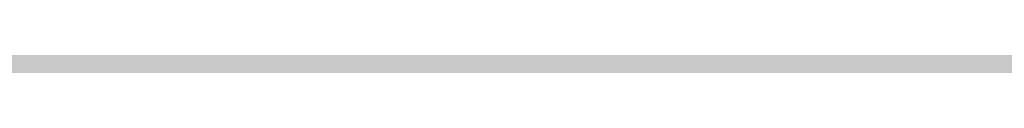
# Model space of a CAD drawing. Units: inches. Extents: x 2091 to 2899, y 967 to 2217.
# Tile 212 of 256: x 2203.2571 to 2203.4104, y 1152.2475 to 1152.2479. Entities that reach past the tile are written whole.
import ezdxf

# ---------------------------------------------------------------- set-up
doc = ezdxf.new("R2010")
doc.units = ezdxf.units.IN
doc.layers.add('A-WALL-PATT', color=141, linetype='Continuous', lineweight=13, true_color=0xadddf7)

msp = doc.modelspace()

# ---------------------------------------------------------------- hatches: boundary and pattern name
at = {"layer": 'A-WALL-PATT'}
h = msp.add_hatch(color=256, dxfattribs=at)
h.dxf.hatch_style = 1
h.paths.add_polyline_path([(2803.1436, 2050.91906), (2203.1436, 2050.91906), (2203.1436, 1090.91906), (2803.1436, 1090.91906)])
h.paths.add_polyline_path([(2635.79885, 1147.54046), (2674.52405, 1147.54046, 0.376086), (2678.52967, 1152.8802), (2678.52967, 1159.55647, 0.333335), (2674.52432, 1163.56185), (2674.52432, 1163.56185), (2674.52432, 1192.93439), (2635.80597, 1192.93439), (2597.08762, 1192.93439), (2597.08762, 1163.56185, 0.333335), (2593.08228, 1159.55647), (2593.08228, 1152.8802, 0.376086), (2597.08789, 1147.54046)], flags=0)
h.paths.add_polyline_path([(2436.01043, 1278.24078, 0.000483), (2435.95264, 1278.21503, -0.001328), (2435.93563, 1278.11169, -0.001711), (2436.11644, 1278.04076, 0.002185)], flags=0)
h.paths.add_polyline_path([(2794.1436, 1143.41906), (2794.1436, 1347.41906), (2543.37017, 1347.41906), (2543.37017, 1351.91906), (2794.1436, 1351.91906), (2794.1436, 1392.71355), (2793.9474, 1392.71355), (2793.9474, 1473.5369), (2794.1436, 1473.5369), (2794.1436, 1531.91906), (2650.1436, 1531.91906), (2650.1436, 1536.41906), (2794.1436, 1536.41906), (2794.1436, 1692.41906), (2609.37561, 1692.41906), (2609.37561, 1644.41906), (2604.87561, 1644.41906), (2604.87561, 1744.91906), (2609.37561, 1744.91906), (2609.37561, 1696.91906), (2794.1436, 1696.91906), (2794.1436, 1780.91906), (2609.6436, 1780.91906), (2493.87561, 1780.91906), (2493.87561, 1785.41906), (2609.6436, 1785.41906), (2794.1436, 1785.41906), (2794.1436, 1847.93882), (2793.95122, 1847.93882), (2793.95122, 1928.76217), (2794.1436, 1928.76217), (2794.1436, 1941.41906), (2614.1436, 1941.41906), (2614.1436, 1821.41906), (2609.6436, 1821.41906), (2609.6436, 1941.41906), (2392.1436, 1941.41906), (2392.1436, 1819.91906), (2387.6436, 1819.91906), (2387.6436, 1941.41906), (2212.1436, 1941.41906), (2212.1436, 1783.91906), (2392.1436, 1783.91906), (2392.1436, 1780.91906), (2212.1436, 1780.91906), (2212.1436, 1629.41906), (2387.6436, 1629.41906), (2387.6436, 1744.91906), (2392.1436, 1744.91906), (2392.1436, 1627.91906), (2317.1436, 1627.91906), (2317.1436, 1551.41906), (2317.1436, 1536.41906), (2459.38359, 1536.41906), (2459.38359, 1602.39648), (2463.88359, 1602.39648), (2463.88359, 1531.91906), (2456.6436, 1531.91906), (2456.6436, 1529.91906), (2452.1436, 1529.91906), (2452.1436, 1531.91906), (2312.6436, 1531.91906), (2312.6436, 1551.41906), (2306.1436, 1551.41906), (2306.1436, 1555.91906), (2308.1436, 1555.91906), (2308.1436, 1551.41906), (2312.6436, 1551.41906), (2312.6436, 1627.91906), (2212.1436, 1627.91906), (2212.1436, 1555.91906), (2270.1436, 1555.91906), (2270.1436, 1551.41906), (2212.1436, 1551.41906), (2212.1436, 1351.91906), (2272.1436, 1351.91906), (2272.1436, 1347.41906), (2212.1436, 1347.41906), (2212.1436, 1275.41906), (2308.1436, 1275.41906), (2308.1436, 1351.91906), (2452.1436, 1351.91906), (2452.1436, 1493.91906), (2456.6436, 1493.91906), (2456.6436, 1347.41906), (2312.6436, 1347.41906), (2312.6436, 1270.91906), (2212.1436, 1270.91906), (2212.1436, 1099.91906), (2281.23752, 1099.91906), (2282.87104, 1110.9138), (2282.00834, 1116.9966), (2278.55774, 1121.4204), (2268.20564, 1128.0562), (2272.08764, 1128.0562), (2273.81294, 1131.927), (2279.42034, 1134.6919), (2285.02784, 1135.2449), (2287.61584, 1137.4568), (2288.04714, 1138.0098), (2289.34114, 1140.7747), (2291.06654, 1139.6687), (2292.36054, 1135.2449), (2295.37984, 1136.9038), (2296.24254, 1135.7979), (2297.10524, 1133.033), (2300.12464, 1138.0098), (2303.14394, 1138.0098), (2304.43794, 1135.7979), (2303.14394, 1133.586), (2306.59464, 1134.6919), (2307.88874, 1133.033), (2310.90804, 1135.2449), (2313.92744, 1134.1389), (2315.62686, 1132.4271), (2308.32004, 1117.5496), (2290.20384, 1109.8079), (2288.90984, 1103.1721), (2289.27231, 1099.91906), (2434.91823, 1099.91906), (2431.59323, 1124.78806), (2429.93023, 1169.55306), (2430.92718, 1240.51969), (2435.65893, 1238.18613), (2437.13523, 1196.55406), (2438.79823, 1143.97306), (2442.67823, 1111.99806), (2446.55823, 1099.91906), (2794.1436, 1099.91906), (2794.1436, 1138.91906), (2548.03245, 1138.91906), (2548.03245, 1143.41906), (2548.03245, 1148.81906), (2546.66846, 1148.03156), (2528.68569, 1179.17862, 0.256256), (2512.03245, 1148.81906), (2512.03245, 1143.41906), (2512.03245, 1138.91906), (2507.53245, 1138.91906), (2507.53245, 1143.41906), (2507.53245, 1148.81906, 0.256256), (2490.8792, 1179.17862), (2472.89644, 1148.03156), (2471.53245, 1148.81906), (2471.53245, 1143.41906), (2467.03245, 1143.41906), (2467.03245, 1269.94579, 0.039061), (2460.90999, 1273.58006), (2467.03245, 1273.58006), (2467.03245, 1286.32536, 0.014511), (2465.21619, 1286.76191), (2467.03245, 1287.05258), (2467.03245, 1323.41906), (2471.53245, 1323.41906), (2471.53245, 1148.81906), (2489.53245, 1179.99597), (2490.89644, 1179.20847), (2490.8792, 1179.17862, -0.256256), (2507.53245, 1148.81906), (2507.53245, 1143.41906), (2512.03245, 1143.41906), (2512.03245, 1148.81906, -0.256256), (2528.68569, 1179.17862), (2528.66846, 1179.20847), (2530.03245, 1179.99597), (2548.03245, 1148.81906), (2548.03245, 1143.41906)], flags=16)
h.paths.add_polyline_path([(2607.76855, 1200.94508), (2607.76855, 1265.03063), (2597.08762, 1281.05201), (2619.78459, 1281.05201), (2627.79528, 1337.12686), (2635.79885, 1337.12686), (2643.81666, 1337.12686), (2651.82736, 1281.05201), (2674.52432, 1281.05201), (2663.8434, 1265.03063), (2663.8434, 1200.94508), (2635.80597, 1200.94508)], flags=0)
edge = h.paths.add_edge_path(flags=0)
edge.add_ellipse((13303.89622, 1272.99872), major_axis=(-10595.31304, 0), ratio=0.84230387009, start_angle=0.628237219, end_angle=0.6465541, ccw=False)
edge.add_ellipse((2711.70045, 1156.85268), major_axis=(2.21977, 0), ratio=0.8423039, start_angle=111.53524, end_angle=180.62824, ccw=False)
edge.add_ellipse((13303.15629, 1272.99872), major_axis=(-10593.02631, 0), ratio=0.84230386954, start_angle=0.528271472, end_angle=0.646554097, ccw=False)
edge.add_line((2710.7646, 1175.3333), (2710.12999, 1175.3333))
edge.add_ellipse((2710.12999, 1176.57978), major_axis=(1.47985, 0), ratio=0.8423039, start_angle=180, end_angle=270, ccw=False)
edge.add_line((2708.65014, 1176.57978), (2708.65014, 1200.78291))
edge.add_ellipse((2710.12999, 1200.78291), major_axis=(1.47985, 0), ratio=0.8423039, start_angle=90, end_angle=180, ccw=False)
edge.add_line((2710.12999, 1202.02939), (2710.46508, 1202.02939))
edge.add_ellipse((13303.15629, 1272.99872), major_axis=(-10593.02631, 0), ratio=0.84230386954, start_angle=-0.090229089, end_angle=0.383866779, ccw=False)
edge.add_ellipse((2710.12999, 1290.92703), major_axis=(-1.47985, 0), ratio=0.8423039, start_angle=0, end_angle=90, ccw=False)
edge.add_line((2708.65014, 1290.92703), (2708.65014, 1315.13017))
edge.add_ellipse((2710.12999, 1315.13017), major_axis=(-1.47985, 0), ratio=0.8423039, start_angle=-90, end_angle=0, ccw=False)
edge.add_line((2710.12999, 1316.37665), (2710.70631, 1316.37665))
edge.add_ellipse((3238.40172, 1296.28957), major_axis=(528.234, 0), ratio=0.84230387, start_angle=176.3495724, end_angle=177.8200497, ccw=False)
edge.add_ellipse((2775.06304, 1071.4507), major_axis=(313.30776, 0), ratio=0.84230387, start_angle=102.1259656, end_angle=103.780529, ccw=False)
edge.add_ellipse((2775.06304, 1078.3057), major_axis=(-305.30289, 0), ratio=0.84230387, start_angle=-79.790461, end_angle=-77.5553727, ccw=False)
edge.add_ellipse((2695.14177, 1541.97538), major_axis=(-250.96022, 0), ratio=0.84230387, start_angle=99.256566, end_angle=102.5549326)
edge.add_line((2741.41033, 1334.21426), (2747.13255, 1337.37848))
edge.add_ellipse((2747.53862, 1336.85748), major_axis=(-0.73992, 0), ratio=0.842304, start_angle=270, end_angle=307.93313, ccw=False)
edge.add_ellipse((2747.53862, 1336.85748), major_axis=(-0.73992, 0), ratio=0.842304, start_angle=232.06687, end_angle=270, ccw=False)
edge.add_line((2747.94469, 1337.37848), (2753.66691, 1334.21426))
edge.add_ellipse((2799.93547, 1541.97538), major_axis=(250.96022, 0), ratio=0.84230387, start_angle=257.4450674, end_angle=260.743434)
edge.add_ellipse((2720.01419, 1078.3057), major_axis=(305.30289, 0), ratio=0.84230387, start_angle=77.5553727, end_angle=79.790461, ccw=False)
edge.add_ellipse((2720.01419, 1071.4507), major_axis=(-313.30776, 0), ratio=0.84230387, start_angle=256.219471, end_angle=257.8740344, ccw=False)
edge.add_ellipse((2256.67551, 1296.28957), major_axis=(-528.234, 0), ratio=0.84230387, start_angle=182.1799503, end_angle=183.6504276, ccw=False)
edge.add_line((2784.37092, 1316.37665), (2784.94725, 1316.37665))
edge.add_ellipse((2784.94725, 1315.13017), major_axis=(1.47985, 0), ratio=0.8423039, start_angle=0, end_angle=90, ccw=False)
edge.add_line((2786.42709, 1315.13017), (2786.42709, 1290.92703))
edge.add_ellipse((2784.94725, 1290.92703), major_axis=(1.47985, 0), ratio=0.8423039, start_angle=270, end_angle=360, ccw=False)
edge.add_ellipse((-7808.07906, 1272.99872), major_axis=(10593.02631, 0), ratio=0.84230386954, start_angle=-0.383866779, end_angle=0.090229089, ccw=False)
edge.add_line((2784.61216, 1202.02939), (2784.94725, 1202.02939))
edge.add_ellipse((2784.94725, 1200.78291), major_axis=(1.47985, 0), ratio=0.8423039, start_angle=0, end_angle=90, ccw=False)
edge.add_line((2786.42709, 1200.78291), (2786.42709, 1176.57978))
edge.add_ellipse((2784.94725, 1176.57978), major_axis=(-1.47985, 0), ratio=0.8423039, start_angle=90, end_angle=180, ccw=False)
edge.add_line((2784.94725, 1175.3333), (2784.31264, 1175.3333))
edge.add_ellipse((-7808.07906, 1272.99872), major_axis=(10593.02631, 0), ratio=0.84230386954, start_angle=-0.618643196, end_angle=-0.528271472, ccw=False)
edge.add_ellipse((2783.37678, 1156.85268), major_axis=(-2.21977, 0), ratio=0.8423039, start_angle=179.37176, end_angle=248.46476, ccw=False)
edge.add_ellipse((-7808.81898, 1272.99872), major_axis=(-10595.31304, 0), ratio=0.84230386576, start_angle=179.353445923, end_angle=179.371762803, ccw=False)
edge.add_ellipse((2780.2973, 1153.50079), major_axis=(-5.24643, 0), ratio=0.8423039, start_angle=90, end_angle=179.35345, ccw=False)
edge.add_line((2780.2973, 1149.08171), (2714.77993, 1149.08171))
edge.add_ellipse((2714.77993, 1153.50079), major_axis=(5.24643, 0), ratio=0.8423039, start_angle=180.64655, end_angle=270, ccw=False)
edge = h.paths.add_edge_path(flags=0)
edge.add_line((2718.18737, 1151.00783), (2718.18737, 1170.47236))
edge.add_ellipse((2721.14706, 1170.47236), major_axis=(-2.95969, 0), ratio=0.8423039, start_angle=-90, end_angle=0, ccw=False)
edge.add_line((2721.14706, 1172.96532), (2773.93017, 1172.96532))
edge.add_ellipse((2773.93017, 1170.47236), major_axis=(-2.95969, 0), ratio=0.8423039, start_angle=180, end_angle=270, ccw=False)
edge.add_line((2776.88987, 1170.47236), (2776.88987, 1151.00783))
edge.add_line((2776.88987, 1151.00783), (2718.18737, 1151.00783))
edge = h.paths.add_edge_path(flags=0)
edge.add_line((2718.18737, 1180.23415), (2718.18737, 1199.05783))
edge.add_ellipse((2747.53862, 1320.39864), major_axis=(147.01792, 0), ratio=0.84230387, start_angle=256.4018653, end_angle=283.5981347)
edge.add_line((2776.88987, 1199.05783), (2776.88987, 1180.23415))
edge.add_ellipse((2747.53862, 1301.57496), major_axis=(147.01792, 0), ratio=0.84230387, start_angle=256.4018653, end_angle=283.5981347, ccw=False)
edge = h.paths.add_edge_path(flags=0)
edge.add_ellipse((13303.15629, 1272.99872), major_axis=(-10591.54646, 0), ratio=0.84230386955, start_angle=0.055594314, end_angle=0.377764194, ccw=False)
edge.add_line((2711.61686, 1262.72171), (2715.66741, 1249.4954))
edge.add_ellipse((6413.89196, 1241.69192), major_axis=(-3698.23616, 0), ratio=0.8423038695, start_angle=-0.12089737, end_angle=0.36407635)
edge.add_line((2715.76104, 1218.19245), (2711.93431, 1203.16736))
edge = h.paths.add_edge_path(flags=0)
edge.add_line((2718.18737, 1251.07457), (2716.00249, 1267.45044))
edge.add_ellipse((2742.15117, 1202.18954), major_axis=(81.77258, 0), ratio=0.84230387, start_angle=94.277421, end_angle=111.8349538, ccw=False)
edge.add_line((2737.00975, 1270.93063), (2758.06748, 1270.93063))
edge.add_ellipse((2752.92606, 1202.18954), major_axis=(81.77258, 0), ratio=0.84230387, start_angle=68.1650462, end_angle=85.722579, ccw=False)
edge.add_line((2779.07475, 1267.45044), (2776.88987, 1251.07457))
edge.add_ellipse((2750.33806, 1187.88536), major_axis=(79.57966, 0), ratio=0.84230387, start_angle=67.2080851, end_angle=85.1299304)
edge.add_line((2756.03466, 1254.74366), (2739.04258, 1254.74366))
edge.add_ellipse((2744.73917, 1187.88536), major_axis=(79.57966, 0), ratio=0.84230387, start_angle=94.8700696, end_angle=112.7919149)
edge = h.paths.add_edge_path(flags=0)
edge.add_line((2783.14293, 1203.16736), (2779.31619, 1218.19245))
edge.add_ellipse((-918.81473, 1241.69192), major_axis=(3698.23616, 0), ratio=0.8423038695, start_angle=-0.36407635, end_angle=0.12089737)
edge.add_line((2779.40983, 1249.4954), (2783.46037, 1262.72171))
edge.add_ellipse((-7808.07906, 1272.99872), major_axis=(-10591.54646, 0), ratio=0.84230386954, start_angle=179.622235806, end_angle=179.944405687, ccw=False)
edge = h.paths.add_edge_path(flags=0)
edge.add_ellipse((2734.20089, 1286.69044), major_axis=(-0.35661, 6.34008), ratio=0.6038336, start_angle=89.002014, end_angle=253.657408, ccw=False)
edge.add_line((2730.369, 1286.54181), (2730.369, 1301.35198))
edge.add_line((2730.369, 1301.35198), (2735.91331, 1305.2148))
edge.add_ellipse((2736.38492, 1304.73456), major_axis=(0.73992, 0), ratio=0.842304, start_angle=90, end_angle=134.48021, ccw=False)
edge.add_line((2736.38492, 1305.3578), (2738.03278, 1305.3578))
edge.add_line((2738.03278, 1305.3578), (2738.03278, 1307.70793))
edge.add_ellipse((2794.20164, 1307.70793), major_axis=(56.16886, 0), ratio=0.84230387, start_angle=150.56143, end_angle=180, ccw=False)
edge.add_ellipse((2700.87559, 1307.70793), major_axis=(-56.16886, 0), ratio=0.84230387, start_angle=180, end_angle=209.43857, ccw=False)
edge.add_line((2757.04445, 1307.70793), (2757.04445, 1305.3578))
edge.add_line((2757.04445, 1305.3578), (2758.69232, 1305.3578))
edge.add_ellipse((2758.69232, 1304.73456), major_axis=(-0.73992, 0), ratio=0.842304, start_angle=225.51979, end_angle=270, ccw=False)
edge.add_line((2759.16392, 1305.2148), (2764.70823, 1301.35198))
edge.add_line((2764.70823, 1301.35198), (2764.70823, 1286.54181))
edge.add_ellipse((2760.87634, 1286.69044), major_axis=(0.35661, 6.34008), ratio=0.6038336, start_angle=106.342592, end_angle=270.997986, ccw=False)
edge.add_line((2757.04445, 1285.79709), (2757.04445, 1307.70793))
edge.add_ellipse((2700.87559, 1307.70793), major_axis=(-56.16886, 0), ratio=0.84230387, start_angle=180, end_angle=209.43857)
edge.add_ellipse((2794.20164, 1307.70793), major_axis=(56.16886, 0), ratio=0.84230387, start_angle=150.56143, end_angle=180)
edge.add_line((2738.03278, 1307.70793), (2738.03278, 1285.79709))
h.paths.add_polyline_path([(2417.81227, 1104.4497), (2413.49227, 1102.5297), (2410.61227, 1103.9697), (2409.17227, 1106.3697), (2407.25227, 1107.3297), (2406.29227, 1109.7297), (2405.33227, 1114.0497), (2405.33227, 1117.8897), (2406.29227, 1120.1297), (2407.25227, 1119.8097), (2408.84832, 1118.32766), (2410.17395, 1119.42417), (2410.21127, 1120.4057), (2411.04073, 1121.41905), (2410.69927, 1119.8587), (2410.17395, 1119.42417), (2410.08845, 1117.17611), (2411.13284, 1116.20632), (2413.97227, 1119.3297), (2416.85227, 1120.7697), (2416.86972, 1120.79878), (2417.03507, 1119.40512), (2417.89621, 1118.14338), (2418.29227, 1118.3697), (2419.54445, 1120.03927), (2419.36092, 1118.38749), (2419.03211, 1119.35615), (2418.39894, 1118.51193), (2419.25227, 1114.5297), (2418.79409, 1107.19879)], flags=0)
h.paths.add_polyline_path([(2508.87017, 1347.41906), (2508.37017, 1347.41906), (2508.37017, 1351.91906), (2508.87017, 1351.91906)], flags=0)
h.paths.add_polyline_path([(2473.37017, 1347.41906), (2472.37017, 1347.41906), (2467.87017, 1347.41906), (2467.87017, 1455.41906), (2472.37017, 1455.41906), (2472.37017, 1352.41906), (2473.37017, 1352.41906)], flags=0)
h.paths.add_polyline_path([(2352.10624, 1217.4462), (2349.22624, 1218.8862), (2347.78624, 1221.2862), (2345.86624, 1222.2462), (2344.90624, 1224.6462), (2343.94624, 1228.9662), (2343.94624, 1232.8062), (2344.90624, 1235.0462), (2345.86624, 1234.7262), (2347.46229, 1233.24415), (2348.78792, 1234.34066), (2348.82524, 1235.3222), (2349.6547, 1236.33555), (2349.31324, 1234.7752), (2348.78792, 1234.34066), (2348.70242, 1232.0926), (2349.74681, 1231.12282), (2352.58624, 1234.2462), (2355.46624, 1235.6862), (2355.48369, 1235.71528), (2355.64904, 1234.32161), (2356.51018, 1233.05988), (2356.90624, 1233.2862), (2358.15842, 1234.95576), (2357.97489, 1233.30398), (2357.64608, 1234.27264), (2357.01291, 1233.42842), (2357.86624, 1229.4462), (2357.40806, 1222.11529), (2356.42624, 1219.3662)], flags=0)
h.paths.add_polyline_path([(2348.2968, 1112.22442), (2347.0138, 1112.31042), (2345.5298, 1114.12742), (2345.7318, 1115.85842), (2346.8118, 1116.98242), (2346.8118, 1114.64642), (2345.8668, 1114.21442), (2346.8798, 1114.30042)], flags=0)
h.paths.add_polyline_path([(2347.0138, 1110.92642), (2346.2718, 1110.49342), (2346.6098, 1111.18642)], flags=0)
h.paths.add_polyline_path([(2345.8668, 1118.19442), (2345.5298, 1117.32942), (2343.7078, 1118.02142), (2344.3828, 1118.62642)], flags=0)
h.paths.add_polyline_path([(2346.6768, 1109.28242), (2346.0698, 1108.07142), (2345.8668, 1110.06142)], flags=0)
h.paths.add_polyline_path([(2345.0568, 1119.75142), (2343.6398, 1119.75142), (2343.9778, 1121.13542)], flags=0)
h.paths.add_polyline_path([(2345.2598, 1116.55042), (2345.1248, 1115.85842), (2344.9218, 1115.68542), (2344.7198, 1116.37742)], flags=0)
h.paths.add_polyline_path([(2345.6648, 1112.31042), (2345.4618, 1111.53242), (2344.0448, 1111.96442), (2344.6518, 1112.57042)], flags=0)
h.paths.add_polyline_path([(2345.1918, 1113.34942), (2344.4498, 1113.86842), (2344.7198, 1114.38742)], flags=0)
h.paths.add_polyline_path([(2344.6518, 1116.80942), (2344.1798, 1115.68542), (2344.6518, 1115.33942), (2343.9098, 1114.90642), (2343.0328, 1115.94442), (2343.6398, 1116.46342)], flags=0)
h.paths.add_polyline_path([(2345.8668, 1106.68642), (2344.9898, 1105.56242), (2344.5168, 1106.60042)], flags=0)
h.paths.add_polyline_path([(2344.8548, 1110.06142), (2344.5168, 1109.28242), (2344.1128, 1109.71542)], flags=0)
h.paths.add_polyline_path([(2344.0448, 1113.52242), (2343.4378, 1113.08942), (2342.7628, 1113.95442)], flags=0)
h.paths.add_polyline_path([(2344.3148, 1111.01242), (2342.9648, 1110.32042), (2342.9648, 1111.09942)], flags=0)
h.paths.add_polyline_path([(2345.1248, 1104.69742), (2344.5848, 1103.74542), (2344.4498, 1104.26442)], flags=0)
h.paths.add_polyline_path([(2342.8298, 1121.22242), (2341.7498, 1120.53042), (2340.5358, 1121.04942), (2340.1308, 1121.82842), (2340.6708, 1122.95242), (2341.1428, 1121.82842), (2341.6148, 1122.00142)], flags=0)
h.paths.add_polyline_path([(2342.9648, 1119.75142), (2343.0328, 1118.45342), (2342.0878, 1118.02142), (2342.0198, 1119.49142)], flags=0)
h.paths.add_polyline_path([(2342.6948, 1116.89642), (2341.9528, 1116.63642), (2342.0198, 1117.32942)], flags=0)
h.paths.add_polyline_path([(2343.0328, 1112.22442), (2342.0198, 1111.79142), (2341.5478, 1112.22442), (2342.3578, 1113.34942)], flags=0)
h.paths.add_polyline_path([(2343.7748, 1104.43742), (2342.6278, 1102.88042), (2342.6948, 1104.61042), (2343.4378, 1105.12942)], flags=0)
h.paths.add_polyline_path([(2342.0198, 1115.07942), (2340.8058, 1115.51242), (2340.9408, 1116.37742)], flags=0)
h.paths.add_polyline_path([(2341.4808, 1120.09742), (2341.4808, 1119.40542), (2341.0758, 1119.57842), (2341.1428, 1120.09742)], flags=0)
h.paths.add_polyline_path([(2341.8178, 1114.47342), (2340.9408, 1113.08942), (2340.8058, 1114.56042)], flags=0)
h.paths.add_polyline_path([(2341.1428, 1118.54042), (2340.9408, 1116.98242), (2339.0508, 1117.67542), (2339.0508, 1118.62642)], flags=0)
h.paths.add_polyline_path([(2342.6948, 1101.66842), (2341.9528, 1101.84142), (2342.5598, 1102.36142)], flags=0)
h.paths.add_polyline_path([(2340.3328, 1119.66542), (2338.4438, 1119.57842), (2337.9038, 1120.35742), (2339.6578, 1120.61642)], flags=0)
h.paths.add_polyline_path([(2340.3328, 1115.33942), (2340.0628, 1113.69542), (2339.3878, 1115.33942)], flags=0)
h.paths.add_polyline_path([(2341.8178, 1103.83142), (2341.5478, 1102.88042), (2341.1428, 1103.65842)], flags=0)
h.paths.add_polyline_path([(2339.0508, 1122.86642), (2337.2958, 1121.82842), (2337.0938, 1123.12542), (2337.7688, 1123.81842)], flags=0)
h.paths.add_polyline_path([(2339.1178, 1121.74142), (2338.8478, 1121.22242), (2338.1738, 1121.04942), (2338.3758, 1121.56842)], flags=0)
h.paths.add_polyline_path([(2339.1858, 1119.31942), (2338.6458, 1118.71342), (2338.2408, 1118.10742), (2338.2408, 1118.88642)], flags=0)
h.paths.add_polyline_path([(2341.1428, 1101.92842), (2340.6028, 1101.23642), (2340.0628, 1101.84142), (2340.6028, 1102.36142)], flags=0)
h.paths.add_polyline_path([(2337.6338, 1117.76142), (2336.6208, 1118.28042), (2337.2958, 1118.97242)], flags=0)
h.paths.add_polyline_path([(2336.8238, 1119.57842), (2334.7988, 1118.97242), (2335.2038, 1120.35742), (2336.5538, 1120.87642)], flags=0)
h.paths.add_polyline_path([(2339.1178, 1100.45742), (2337.3638, 1100.54342), (2336.7558, 1101.23642)], flags=0)
h.paths.add_polyline_path([(2336.3508, 1122.43342), (2336.0138, 1121.91442), (2334.9338, 1122.43342), (2334.5288, 1123.47142), (2335.7438, 1122.77942)], flags=0)
h.paths.add_polyline_path([(2334.7318, 1120.87642), (2334.2588, 1120.35742), (2334.0568, 1120.78942), (2334.5968, 1121.30842)], flags=0)
h.paths.add_polyline_path([(2334.4618, 1122.17442), (2332.5718, 1121.30842), (2331.3568, 1122.17442), (2332.0998, 1122.86642)], flags=0)
h.paths.add_polyline_path([(2334.2588, 1118.54042), (2333.3818, 1118.45342), (2333.6518, 1119.31942)], flags=0)
h.paths.add_polyline_path([(2335.5418, 1102.27442), (2334.1918, 1102.62042), (2335.2718, 1103.31242)], flags=0)
h.paths.add_polyline_path([(2332.7068, 1119.66542), (2331.6948, 1120.44342), (2332.5048, 1120.78942)], flags=0)
h.paths.add_polyline_path([(2334.7318, 1101.14942), (2333.5168, 1101.58242), (2333.9888, 1101.75542)], flags=0)
h.paths.add_polyline_path([(2332.6398, 1116.63642), (2331.0868, 1116.29042), (2331.9648, 1118.19442)], flags=0)
h.paths.add_polyline_path([(2330.7498, 1121.56842), (2330.2768, 1120.27042), (2328.5228, 1119.31942), (2328.9948, 1121.04942)], flags=0)
h.paths.add_polyline_path([(2330.7498, 1118.62642), (2330.0078, 1117.50242), (2329.8728, 1118.02142)], flags=0)
h.paths.add_polyline_path([(2332.0998, 1102.36142), (2330.5468, 1102.01442), (2331.6948, 1102.96642)], flags=0)
h.paths.add_polyline_path([(2329.5348, 1113.60842), (2329.0628, 1112.31042), (2328.5898, 1113.34942)], flags=0)
h.paths.add_polyline_path([(2328.3878, 1117.84842), (2327.5098, 1116.55042), (2327.1728, 1117.76142)], flags=0)
h.paths.add_polyline_path([(2329.7378, 1106.51342), (2329.5348, 1105.30242), (2328.2528, 1106.08142)], flags=0)
h.paths.add_polyline_path([(2328.6578, 1114.38742), (2328.0498, 1114.12742), (2328.3198, 1114.90642)], flags=0)
h.paths.add_polyline_path([(2328.3198, 1112.22442), (2327.1058, 1112.13742), (2326.7008, 1112.65642)], flags=0)
h.paths.add_polyline_path([(2326.9028, 1115.25242), (2326.7008, 1114.12742), (2325.2158, 1113.60842), (2326.0928, 1115.33942)], flags=0)
h.paths.add_polyline_path([(2326.6328, 1108.33042), (2326.0928, 1107.37942), (2325.8908, 1108.50342), (2326.4978, 1109.10942)], flags=0)
h.paths.add_polyline_path([(2615.1436, 1531.91906), (2609.6436, 1531.91906), (2609.6436, 1620.41906), (2614.1436, 1620.41906), (2614.1436, 1536.41906), (2615.1436, 1536.41906)], flags=0)
h.paths.add_polyline_path([(2545.1436, 1563.41906), (2464.1436, 1563.41906), (2464.1436, 1632.41906), (2509.1436, 1632.41906), (2509.1436, 1627.91906), (2509.1436, 1603.91906), (2468.6436, 1603.91906), (2468.6436, 1567.91906), (2540.6436, 1567.91906), (2540.6436, 1591.91906), (2545.1436, 1591.91906)], flags=0)
h.paths.add_polyline_path([(2388.96905, 1549.98573), (2357.43418, 1549.98573), (2357.43418, 1623.36078), (2399.36278, 1623.36078), (2435.68947, 1623.36078), (2435.59255, 1602.55927), (2435.59255, 1602.39648), (2388.96905, 1602.39648)], flags=0)
h.paths.add_polyline_path([(2388.88063, 1555.80915), (2374.90443, 1555.80915), (2374.90443, 1600.57156), (2374.90443, 1615.45765), (2406.35088, 1615.45765), (2406.35088, 1618.93943), (2412.17429, 1615.45765), (2406.35088, 1611.97586), (2406.35088, 1615.45765), (2388.88063, 1615.45765)], flags=0)
h.paths.add_polyline_path([(2568.87561, 1644.41906), (2453.37561, 1644.41906), (2453.37561, 1785.41906), (2457.87561, 1785.41906), (2457.87561, 1648.91906), (2568.87561, 1648.91906)], flags=0)
h.paths.add_polyline_path([(2212.1436, 1945.91906), (2212.1436, 2041.91906), (2794.1436, 2041.91906), (2794.1436, 1945.91906)], flags=16)
h.paths.add_polyline_path([(2271.08273, 1964.31724), (2776.85297, 1964.31724), (2776.85297, 2037.16962), (2271.08273, 2037.16962)], flags=8)
h.paths.add_polyline_path([(2380.64929, 1536.82414), (2461.04081, 1536.82414), (2461.04081, 1554.65259), (2380.64929, 1554.65259)], flags=8)
h.paths.add_polyline_path([(2240.75571, 1609.72545), (2309.18583, 1609.72545), (2309.18583, 1617.6982), (2240.75571, 1617.6982)], flags=8)
h.paths.add_polyline_path([(2212.67726, 1313.5041), (2282.59152, 1313.5041), (2282.59152, 1322.74524), (2212.67726, 1322.74524)], flags=8)
h.paths.add_polyline_path([(2457.11198, 1114.77857), (2558.48158, 1114.77857), (2558.48158, 1142.21968), (2457.11198, 1142.21968)], flags=8)
h.paths.add_polyline_path([(2473.44234, 1273.01007), (2604.64123, 1273.01007), (2604.64123, 1318.34693), (2473.44234, 1318.34693)], flags=8)
h.paths.add_polyline_path([(2638.8763, 1626.97743), (2684.25037, 1627.97674), (2684.03848, 1637.59749), (2638.66442, 1636.59819)], flags=8)
h.paths.add_polyline_path([(2537.59055, 1453.79345), (2628.38955, 1453.79345), (2628.38955, 1475.34481), (2537.59055, 1475.34481)], flags=8)
h.paths.add_polyline_path([(2504.13764, 1714.6324), (2554.64719, 1714.6324), (2554.64719, 1730.23771), (2504.13764, 1730.23771)], flags=8)
h.paths.add_polyline_path([(2487.50118, 1575.65187), (2535.09712, 1575.65187), (2535.09712, 1598.37765), (2487.50118, 1598.37765)], flags=8)
h.paths.add_polyline_path([(2709.0994, 1735.71028), (2740.0166, 1735.71028), (2740.0166, 1749.93764), (2709.0994, 1749.93764)], flags=8)
h.paths.add_polyline_path([(2442.43842, 1792.17166), (2564.72884, 1792.17166), (2564.72884, 1842.00016), (2442.43842, 1842.00016)], flags=8)
h.paths.add_polyline_path([(2655.8158, 1809.64408), (2789.52014, 1806.6938), (2790.08498, 1832.29164), (2656.38064, 1835.24192)], flags=8)
h.paths.add_polyline_path([(2234.8427, 1797.72014), (2368.59285, 1794.76885), (2369.16072, 1820.50413), (2235.41056, 1823.45542)], flags=8)
h.paths.add_polyline_path([(2245.13847, 1644.00633), (2398.42773, 1640.6239), (2398.99484, 1666.32482), (2245.70557, 1669.70725)], flags=8)
h.paths.add_polyline_path([(2306.14285, 1431.16852), (2413.76831, 1428.79369), (2414.33315, 1454.39153), (2306.70768, 1456.76636)], flags=8)
h.paths.add_polyline_path([(2306.83458, 1458.23314), (2393.38048, 1456.32345), (2393.93281, 1481.35436), (2307.38691, 1483.26405)], flags=8)

doc.saveas('drawing.dxf')
